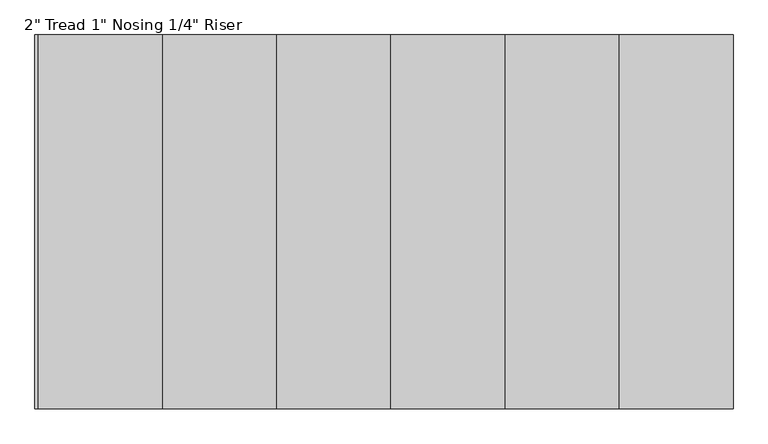
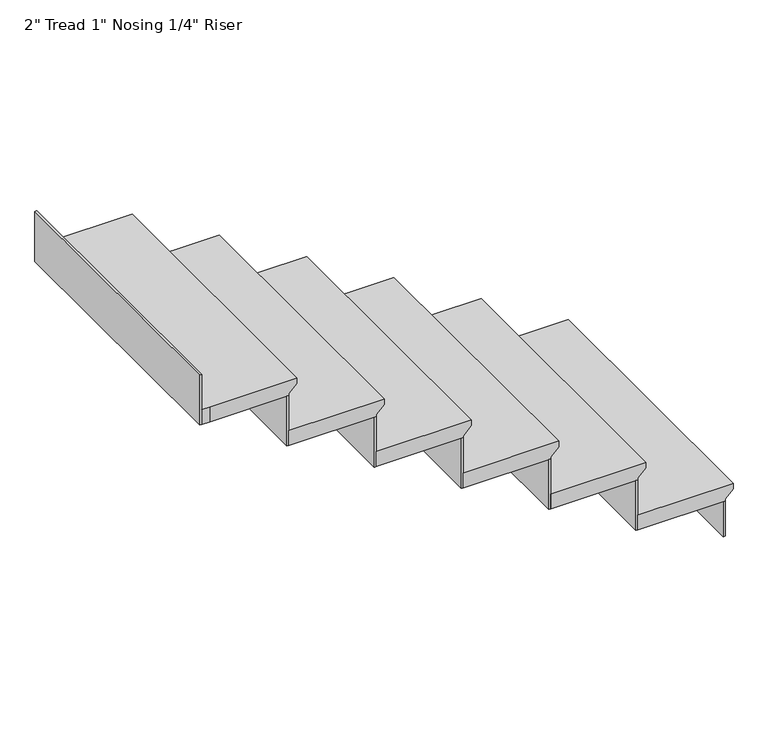
"""IFC4 building model written with IfcOpenShell, lengths in millimetres: stair flight geometry."""

from ifc_helpers import new_model, si_unit, origin, place, context, project, spatial, faceted_brep, source, transform, mapped, element, save


def stair_flight_0804820e(model_context):
    return source(origin(), model_context, "Body", "Brep", [
        faceted_brep([(-3322.4601025, -2869.057314, 455.0833333), (-3322.4601025, -2869.057314, 474.1333333), (-3322.4601025, -3783.457314, 474.1333333), (-3322.4601025, -3783.457314, 455.0833333), (-3347.8601025, -2869.057314, 429.6833333), (-3347.8601025, -3783.457314, 429.6833333), (-3627.2601025, -2869.057314, 474.1333333), (-3627.2601025, -3783.457314, 474.1333333), (-3347.8601025, -3783.457314, 423.3333333), (-3627.2601025, -3783.457314, 423.3333333), (-3627.2601025, -2869.057314, 423.3333333), (-3347.8601025, -2869.057314, 423.3333333)], [[[0, 1, 2, 3]], [[4, 0, 3, 5]], [[2, 1, 6, 7]], [[8, 9, 10, 11]], [[2, 7, 9, 8, 5, 3]], [[8, 11, 4, 5]], [[6, 1, 0, 4, 11, 10]], [[7, 6, 10, 9]]]),
        faceted_brep([(-3347.8601025, -2869.057314, 423.3333333), (-3347.8601025, -2869.057314, 304.8), (-3354.2101025, -2869.057314, 304.8), (-3354.2101025, -2869.057314, 423.3333333), (-3347.8601025, -3783.457314, 423.3333333), (-3354.2101025, -3783.457314, 423.3333333), (-3354.2101025, -3783.457314, 304.8), (-3347.8601025, -3783.457314, 304.8)], [[[0, 1, 2, 3]], [[4, 5, 6, 7]], [[1, 0, 4, 7]], [[2, 1, 7, 6]], [[3, 2, 6, 5]], [[0, 3, 5, 4]]]),
        faceted_brep([(-3627.2601025, -2869.057314, 592.6666667), (-3627.2601025, -2869.057314, 423.3333333), (-3633.6101025, -2869.057314, 423.3333333), (-3633.6101025, -2869.057314, 592.6666667), (-3627.2601025, -3783.457314, 592.6666667), (-3633.6101025, -3783.457314, 592.6666667), (-3633.6101025, -3783.457314, 423.3333333), (-3627.2601025, -3783.457314, 423.3333333)], [[[0, 1, 2, 3]], [[4, 5, 6, 7]], [[1, 0, 4, 7]], [[2, 1, 7, 6]], [[3, 2, 6, 5]], [[0, 3, 5, 4]]]),
        faceted_brep([(-3601.8601025, -3783.457314, 643.4666667), (-3601.8601025, -2869.057314, 643.4666667), (-3906.6601025, -2869.057314, 643.4666667), (-3906.6601025, -3783.457314, 643.4666667), (-3627.2601025, -3783.457314, 592.6666667), (-3906.6601025, -3783.457314, 592.6666667), (-3906.6601025, -2869.057314, 592.6666667), (-3627.2601025, -2869.057314, 592.6666667), (-3627.2601025, -3783.457314, 599.0166667), (-3601.8601025, -3783.457314, 624.4166667), (-3627.2601025, -2869.057314, 599.0166667), (-3601.8601025, -2869.057314, 624.4166667)], [[[0, 1, 2, 3]], [[4, 5, 6, 7]], [[0, 3, 5, 4, 8, 9]], [[4, 7, 10, 8]], [[2, 1, 11, 10, 7, 6]], [[3, 2, 6, 5]], [[11, 1, 0, 9]], [[10, 11, 9, 8]]]),
        faceted_brep([(-3906.6601025, -2869.057314, 762.0), (-3906.6601025, -2869.057314, 592.6666667), (-3913.0101025, -2869.057314, 592.6666667), (-3913.0101025, -2869.057314, 762.0), (-3906.6601025, -3783.457314, 762.0), (-3913.0101025, -3783.457314, 762.0), (-3913.0101025, -3783.457314, 592.6666667), (-3906.6601025, -3783.457314, 592.6666667)], [[[0, 1, 2, 3]], [[4, 5, 6, 7]], [[1, 0, 4, 7]], [[2, 1, 7, 6]], [[3, 2, 6, 5]], [[0, 3, 5, 4]]]),
        faceted_brep([(-3881.2601025, -3783.457314, 812.8), (-3881.2601025, -2869.057314, 812.8), (-4186.0601025, -2869.057314, 812.8), (-4186.0601025, -3783.457314, 812.8), (-3906.6601025, -3783.457314, 762.0), (-4186.0601025, -3783.457314, 762.0), (-4186.0601025, -2869.057314, 762.0), (-3906.6601025, -2869.057314, 762.0), (-3906.6601025, -3783.457314, 768.35), (-3881.2601025, -3783.457314, 793.75), (-3906.6601025, -2869.057314, 768.35), (-3881.2601025, -2869.057314, 793.75)], [[[0, 1, 2, 3]], [[4, 5, 6, 7]], [[0, 3, 5, 4, 8, 9]], [[4, 7, 10, 8]], [[2, 1, 11, 10, 7, 6]], [[3, 2, 6, 5]], [[11, 1, 0, 9]], [[10, 11, 9, 8]]]),
        faceted_brep([(-4186.0601025, -2869.057314, 931.3333333), (-4186.0601025, -2869.057314, 762.0), (-4192.4101025, -2869.057314, 762.0), (-4192.4101025, -2869.057314, 931.3333333), (-4186.0601025, -3783.457314, 931.3333333), (-4192.4101025, -3783.457314, 931.3333333), (-4192.4101025, -3783.457314, 762.0), (-4186.0601025, -3783.457314, 762.0)], [[[0, 1, 2, 3]], [[4, 5, 6, 7]], [[1, 0, 4, 7]], [[2, 1, 7, 6]], [[3, 2, 6, 5]], [[0, 3, 5, 4]]]),
        faceted_brep([(-4160.6601025, -3783.457314, 982.1333333), (-4160.6601025, -2869.057314, 982.1333333), (-4465.4601025, -2869.057314, 982.1333333), (-4465.4601025, -3783.457314, 982.1333333), (-4186.0601025, -3783.457314, 931.3333333), (-4465.4601025, -3783.457314, 931.3333333), (-4465.4601025, -2869.057314, 931.3333333), (-4186.0601025, -2869.057314, 931.3333333), (-4186.0601025, -3783.457314, 937.6833333), (-4160.6601025, -3783.457314, 963.0833333), (-4186.0601025, -2869.057314, 937.6833333), (-4160.6601025, -2869.057314, 963.0833333)], [[[0, 1, 2, 3]], [[4, 5, 6, 7]], [[0, 3, 5, 4, 8, 9]], [[4, 7, 10, 8]], [[2, 1, 11, 10, 7, 6]], [[3, 2, 6, 5]], [[11, 1, 0, 9]], [[10, 11, 9, 8]]]),
        faceted_brep([(-4465.4601025, -2869.057314, 1100.6666667), (-4465.4601025, -2869.057314, 931.3333333), (-4471.8101025, -2869.057314, 931.3333333), (-4471.8101025, -2869.057314, 1100.6666667), (-4465.4601025, -3783.457314, 1100.6666667), (-4471.8101025, -3783.457314, 1100.6666667), (-4471.8101025, -3783.457314, 931.3333333), (-4465.4601025, -3783.457314, 931.3333333)], [[[0, 1, 2, 3]], [[4, 5, 6, 7]], [[1, 0, 4, 7]], [[2, 1, 7, 6]], [[3, 2, 6, 5]], [[0, 3, 5, 4]]]),
        faceted_brep([(-4440.0601025, -3783.457314, 1151.4666667), (-4440.0601025, -2869.057314, 1151.4666667), (-4744.8601025, -2869.057314, 1151.4666667), (-4744.8601025, -3783.457314, 1151.4666667), (-4465.4601025, -3783.457314, 1100.6666667), (-4744.8601025, -3783.457314, 1100.6666667), (-4744.8601025, -2869.057314, 1100.6666667), (-4465.4601025, -2869.057314, 1100.6666667), (-4465.4601025, -3783.457314, 1107.0166667), (-4440.0601025, -3783.457314, 1132.4166667), (-4465.4601025, -2869.057314, 1107.0166667), (-4440.0601025, -2869.057314, 1132.4166667)], [[[0, 1, 2, 3]], [[4, 5, 6, 7]], [[0, 3, 5, 4, 8, 9]], [[4, 7, 10, 8]], [[2, 1, 11, 10, 7, 6]], [[3, 2, 6, 5]], [[11, 1, 0, 9]], [[10, 11, 9, 8]]]),
        faceted_brep([(-5024.2601025, -2869.057314, 1439.3333333), (-5024.2601025, -2869.057314, 1270.0), (-5030.6101025, -2869.057314, 1270.0), (-5030.6101025, -2869.057314, 1439.3333333), (-5024.2601025, -3783.457314, 1439.3333333), (-5030.6101025, -3783.457314, 1439.3333333), (-5030.6101025, -3783.457314, 1270.0), (-5024.2601025, -3783.457314, 1270.0)], [[[0, 1, 2, 3]], [[4, 5, 6, 7]], [[1, 0, 4, 7]], [[2, 1, 7, 6]], [[3, 2, 6, 5]], [[0, 3, 5, 4]]]),
        faceted_brep([(-4744.8601025, -2869.057314, 1270.0), (-4744.8601025, -2869.057314, 1100.6666667), (-4751.2101025, -2869.057314, 1100.6666667), (-4751.2101025, -2869.057314, 1270.0), (-4744.8601025, -3783.457314, 1270.0), (-4751.2101025, -3783.457314, 1270.0), (-4751.2101025, -3783.457314, 1100.6666667), (-4744.8601025, -3783.457314, 1100.6666667)], [[[0, 1, 2, 3]], [[4, 5, 6, 7]], [[1, 0, 4, 7]], [[2, 1, 7, 6]], [[3, 2, 6, 5]], [[0, 3, 5, 4]]]),
        faceted_brep([(-5024.2601025, -3783.457314, 1320.8), (-4998.8601025, -3783.457314, 1320.8), (-4719.4601025, -3783.457314, 1320.8), (-4719.4601025, -2869.057314, 1320.8), (-4998.8601025, -2869.057314, 1320.8), (-5024.2601025, -2869.057314, 1320.8), (-4998.8601025, -3783.457314, 1270.0), (-5024.2601025, -3783.457314, 1270.0), (-5024.2601025, -2869.057314, 1270.0), (-4998.8601025, -2869.057314, 1270.0), (-4744.8601025, -2869.057314, 1270.0), (-4744.8601025, -3783.457314, 1270.0), (-4744.8601025, -3783.457314, 1276.35), (-4719.4601025, -3783.457314, 1301.75), (-4744.8601025, -2869.057314, 1276.35), (-4719.4601025, -2869.057314, 1301.75)], [[[0, 1, 2, 3, 4, 5]], [[6, 7, 8, 9, 10, 11]], [[1, 0, 7, 6]], [[2, 1, 6, 11, 12, 13]], [[11, 10, 14, 12]], [[4, 3, 15, 14, 10, 9]], [[5, 4, 9, 8]], [[0, 5, 8, 7]], [[15, 3, 2, 13]], [[14, 15, 13, 12]]]),
    ])


if __name__ == "__main__":
    model = new_model("IFC4")
    model_context = context("Model", 3, world=origin())
    ifc_project = project(units=[si_unit("LENGTHUNIT", "METRE", prefix="MILLI")], contexts=[model_context])
    site = spatial("IfcSite", under=ifc_project)
    building = spatial("IfcBuilding", under=site)
    placement = place(None, origin())
    stair_flight_shape = stair_flight_0804820e(model_context)
    element("IfcStairFlight", 1, ObjectType="2\" Tread 1\" Nosing 1/4\" Riser", at=placement, inside=building, context=model_context, shape_type="MappedRepresentation", body=[
        mapped(stair_flight_shape, transform((0.0, 0.0, 0.0), x_axis=(1.0, 0.0, 0.0), y_axis=(0.0, 1.0, 0.0), z_axis=(0.0, 0.0, 1.0))),
    ])
    save(model, "model.ifc")
